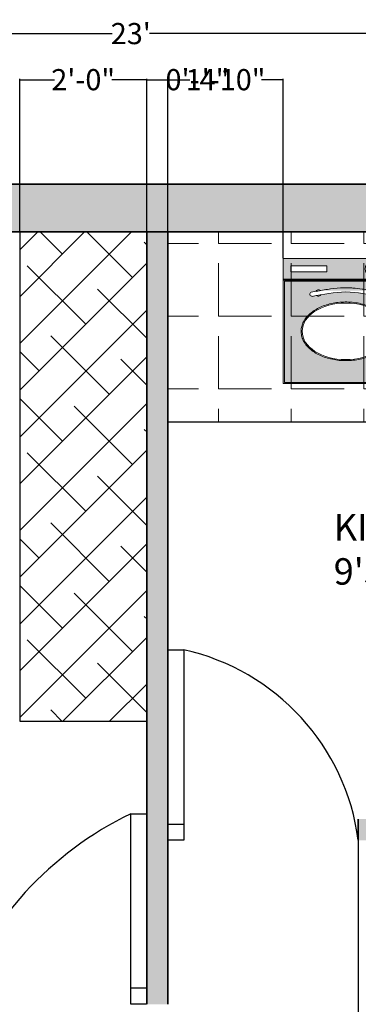
# Model space of a CAD drawing. Units: inches. Extents: x 490 to 851, y 299 to 716.
# Tile 3 of 3: x 664 to 728, y 530 to 716. Entities that reach past the tile are written whole.
import ezdxf

# ---------------------------------------------------------------- set-up
doc = ezdxf.new("R2010")
doc.units = ezdxf.units.IN
doc.header["$MEASUREMENT"] = 0
for name, color, linetype, lineweight in [('A-ANNO-DIMS', 2, 'Continuous', 18), ('A-AREA-IDEN', 7, 'Continuous', 25), ('A-DOOR', 3, 'Continuous', 25), ('A-EQPM', 8, 'Continuous', 18), ('A-EQPM-PATT', 9, 'Continuous', 13), ('A-FLOR-CASE', 40, 'Continuous', 25), ('A-FLOR-CASE-PATT', 9, 'Continuous', 13), ('A-WALL', 7, 'Continuous', 35), ('A-WALL-PATT', 1, 'Continuous', 13)]:
    doc.layers.add(name, color=color, linetype=linetype, lineweight=lineweight)
doc.styles.get("Standard").update_dxf_attribs({"font": 'arial.ttf'})
doc.dimstyles.get("Standard").update_dxf_attribs({"dimtxt": 4, "dimasz": 0.18, "dimexe": 0.18, "dimexo": 0.0625, "dimgap": 0.09, "dimtad": 0, "dimtih": 1, "dimtoh": 1, "dimdec": 0, "dimrnd": 6, "dimzin": 0, "dimdsep": 46, "dimlunit": 3, "dimtxsty": 'Standard', "dimcen": 0.09, "dimadec": 0, "dimazin": 0, "dimtfac": 1, "dimtdec": 0, "dimtofl": 0, "dimtmove": 0, "dimatfit": 3, "dimfxl": 1, "dimtolj": 1, "dimtzin": 0, "dimarcsym": 0})

# ---------------------------------------------------------------- blocks, each defined once
blk = doc.blocks.new('A$C7E884C79')
for p, q in [((-1.70119819813e-05, 1.5003966837e-05), (-1.70119419636e-05, 600.0000150039222)), ((-1.70119419636e-05, 600.0000150039222), (-1.70119819813e-05, 1.5003966837e-05)), ((-1.70119419636e-05, 600.0000150039222), (599.9999829879742, 600.0000150039077)), ((599.9999829879742, 600.0000150039077), (599.9999829880543, 1.5003966837e-05)), ((599.9999829880543, 1.5003966837e-05), (599.9999829879742, 600.0000150039077)), ((599.9999829879742, 600.0000150039077), (599.9999829879742, 450.0000150039659)), ((599.9999829879742, 600.0000150039077), (599.999982988058, 500.0000150039222)), ((599.999982988058, 500.0000150039222), (-1.70119383256e-05, 500.0000150039368)), ((599.999982988058, 495.0000150039441), (-1.70119019458e-05, 495.0000150039368)), ((599.999982988058, 500.0000150039222), (599.9999829880543, 1.5003966837e-05)), ((-1.70119819813e-05, 1.5003966837e-05), (599.9999829880543, 1.5003966837e-05))]:
    blk.add_line(p, q)
for points in [[(36.4219297853997, 564.739244228137), (208.9464086602384, 564.7392442281297), (208.9464086601583, 535.2607857798894), (36.4219297853997, 535.2607857798894)], [(4.999982988054398, 490.0000150040023), (594.999982988018, 490.0000150039513), (594.999982988018, 5.000015003966836), (4.999982987974362, 5.000015003930457)]]:
    blk.add_lwpolyline(points, close=True)
for centre, radius in [((419.341129777058, 550.0000150039514), 27.0465612830012), ((513.9038640534054, 550.0000150040095), 27.0465612830012), ((419.341129777058, 550.0000150039514), 17.0465612830012), ((513.9038640534054, 550.0000150040095), 17.0465612830012)]:
    blk.add_circle(centre, radius)
for centre, radius, start, end in [((137.2371143128039, 427.9571012842962), 9.99999999999936, 107.9829144627732, 276.9581094476087), ((168.4662399462322, 434.1738953022822), 14.99999999999999, 50.78880560725227, 150.3670062790382), ((168.4662399462322, 434.1738953022822), 14.99999999999999, 234.0164507050499, 327.1412143486447), ((431.5337276184946, 434.1738953023768), 14.99999999999999, 212.858785649389, 305.9835492949501), ((431.5337276184946, 434.1738953023768), 14.99999999999999, 29.63299372096182, 129.2111943927477), ((462.7628532516318, 427.957101284347), 9.99999999999936, 263.0418905523912, 72.01708553722673)]:
    blk.add_arc(centre, radius, start, end)
blk.add_ellipse((299.9999829880799, 250.0000150039296), major_axis=(-209.5453259160858, -5.8e-15), ratio=0.6483519184224599)
for points, knots in [([(134.1497789577479, 437.4685875095702), (144.6082166758169, 439.5062024863827), (155.1126203912208, 441.5529426086532), (185.9929094715517, 447.3437385568786), (206.494733029569, 450.9047119657725), (247.8674864836758, 456.3761860351832), (268.7408772092858, 458.286932131693), (293.5357101192494, 458.8504522635657), (297.2767330304487, 458.8901691064702), (304.7624299796444, 458.8727062536881), (308.4995762127364, 458.8160495901202), (319.6935092446511, 458.5127217792715), (327.132745431325, 458.1327232394569), (349.3790513168205, 456.541815341955), (364.1144689435605, 454.8805655177448), (399.790008761498, 449.8898845417889), (420.6328031065277, 446.1500348981672), (449.5099892856014, 440.6522069539087), (457.6940766911502, 439.0576405788188), (465.8501870183317, 437.4685875095119)], [0, 0, 0, 0, 31.63886493985545, 31.63886493985545, 92.6001428223882, 92.6001428223882, 153.561420704921, 153.561420704921, 164.3676472469802, 164.3676472469802, 175.1738737890395, 175.1738737890395, 196.786326873158, 196.786326873158, 240.011233041395, 240.011233041395, 302.0992006983722, 302.0992006983722, 326.7730650015291, 326.7730650015291, 326.7730650015291, 326.7730650015291]), ([(85.4546570720122, 250.000015003995), (85.45465707196854, 244.8170777658043), (85.88822561246344, 239.6342308201456), (88.02000493869853, 226.9220552357911), (90.21816192173355, 219.4365483580441), (96.38934370677816, 204.8396118246929), (100.3615888692657, 197.7281744404427), (109.949488846185, 184.0573372099134), (115.5648436689007, 177.4976038454224), (128.2787075515953, 165.0792487628459), (135.3771921305961, 159.2204529245464), (150.8720546014374, 148.3331296320939), (159.2684172301451, 143.3046103743872), (177.1485118738346, 134.1894280664528), (186.6321541176294, 130.1028504448732), (206.452394453896, 122.9637707452166), (216.7888352855625, 119.9113613978661), (238.0601333966843, 114.9105694415302), (248.9947899629697, 112.9622577759255), (271.1933164569673, 110.2148003270667), (282.4569621843111, 109.4156943254311), (305.0360465127196, 108.9852871540024), (316.3512522399324, 109.3539922337331), (338.7547296880475, 111.250649079022), (349.842772469201, 112.7785733309465), (371.5188673051307, 116.9582324470866), (382.1067079762179, 119.6099073260157), (402.521673323441, 125.9760737243086), (412.3486219806691, 129.6904786132982), (430.9992961862953, 138.0977836687561), (439.8229044345789, 142.7905902191232), (456.2471036538445, 153.0498538677457), (463.8476543751239, 158.616262825697), (477.6310685340795, 170.4997415048819), (483.8139313680366, 176.8169072710916), (494.5927765360757, 190.0604633081639), (499.1886010545786, 196.9871541335851), (506.6510537532812, 211.2839776396031), (509.5170666792983, 218.6543269104914), (513.4150547302415, 233.6388937332849), (514.4461961801352, 241.2525613148282), (514.6307693529524, 256.4928783461756), (513.7841458961847, 264.1183282945521), (510.2477897096396, 279.1482905806288), (507.5588601688614, 286.5521574531694), (500.4381704066108, 300.9341605102481), (496.0070741749878, 307.9124682590946), (485.5423204980033, 321.2743467604842), (479.5088542609591, 327.6582316730155), (466.0064121881987, 339.6881924907093), (458.5374402723464, 345.3343844510992), (442.356079099205, 355.7645443168249), (433.643722825036, 360.5484732858849), (415.1928234087136, 369.1474950443399), (405.4543904653837, 372.9624956318466), (385.1916535080673, 379.5371793190816), (374.6675208302404, 382.2967738713005), (353.0924824455687, 386.6971874674664), (342.0417855184496, 388.3379435140769), (319.6857084956864, 390.4625844960347), (308.380556257187, 390.9464386215868), (285.7940339416527, 390.7459687177425), (274.5128969021971, 390.0616475992965), (252.2522801997875, 387.5407311810659), (241.273026189534, 385.704172406523), (219.886530266871, 380.921302532438), (209.4794921704815, 377.9750595404139), (189.4937597145654, 371.0403800096638), (179.9152279588161, 367.0520348783057), (161.8232383307077, 358.1233102125143), (153.3098778178173, 353.1830191051149), (137.5613657555441, 342.4603322407738), (130.3262354594117, 336.6779568452357), (117.3219427482508, 324.3988645588861), (111.5527951950935, 317.9019950986867), (101.6427302403026, 304.3410831906103), (97.50207040229724, 297.2767107389691), (90.98281377420064, 282.7548846949166), (88.60495846102276, 275.2973569409469), (86.02335275324731, 261.8687924363285), (85.45465707200856, 255.934491795876), (85.4546570720122, 250.000015003995)], [0, 0, 0, 0, 0.1083005230516948, 0.1083005230516948, 0.2675342177864238, 0.2675342177864238, 0.4267679125211527, 0.4267679125211527, 0.5860016072558816, 0.5860016072558816, 0.7452353019906105, 0.7452353019906105, 0.9044689967253393, 0.9044689967253393, 1.063702691460068, 1.063702691460068, 1.222936386194797, 1.222936386194797, 1.382170080929526, 1.382170080929526, 1.541403775664254, 1.541403775664254, 1.700637470398983, 1.700637470398983, 1.859871165133712, 1.859871165133712, 2.019104859868441, 2.019104859868441, 2.17833855460317, 2.17833855460317, 2.337572249337898, 2.337572249337898, 2.496805944072627, 2.496805944072627, 2.656039638807356, 2.656039638807356, 2.815273333542085, 2.815273333542085, 2.974507028276814, 2.974507028276814, 3.133740723011543, 3.133740723011543, 3.292974417746271, 3.292974417746271, 3.452208112481, 3.452208112481, 3.611441807215729, 3.611441807215729, 3.770675501950458, 3.770675501950458, 3.929909196685187, 3.929909196685187, 4.089142891419916, 4.089142891419916, 4.248376586154645, 4.248376586154645, 4.407610280889374, 4.407610280889374, 4.566843975624102, 4.566843975624102, 4.726077670358831, 4.726077670358831, 4.88531136509356, 4.88531136509356, 5.044545059828289, 5.044545059828289, 5.203778754563018, 5.203778754563018, 5.363012449297746, 5.363012449297746, 5.522246144032475, 5.522246144032475, 5.681479838767204, 5.681479838767204, 5.840713533501933, 5.840713533501933, 5.999947228236662, 5.999947228236662, 6.15918092297139, 6.15918092297139, 6.283185307179586, 6.283185307179586, 6.283185307179586, 6.283185307179586])]:
    blk.add_open_spline(points, degree=3, knots=knots)
blk.add_open_spline([(137.9744605147498, 417.8376983042863), (191.9829680058602, 428.3601631990827), (299.999982988136, 449.4050929886863), (408.016997970407, 428.360163199051), (462.0255054615699, 417.837698304228)], degree=3)
blk = doc.blocks.new('*D102')
at = {"layer": 'A-ANNO-DIMS', "color": 0, "lineweight": -2, "transparency": 16777216}
for p, q in [((546.6878542437281, 685.0194991519433), (546.6878542437281, 713.5977998437985)), ((546.867854243728, 713.4177998437985), (681.1694777089394, 713.4177998437985)), ((822.507854243728, 713.4177998437985), (688.2062307785166, 713.4177998437985)), ((822.687854243728, 685.0194991519433), (822.687854243728, 713.5977998437985))]:
    blk.add_line(p, q, dxfattribs=at)
at = {"layer": 'A-ANNO-DIMS', "color": 0, "transparency": 16777216}
for points in [[(546.867854243728, 713.4477998437985), (546.867854243728, 713.3877998437985), (546.6878542437281, 713.4177998437985)], [(822.507854243728, 713.4477998437985), (822.507854243728, 713.3877998437985), (822.687854243728, 713.4177998437985)]]:
    blk.add_solid(points, dxfattribs=at)
at = {"layer": 'Defpoints', "color": 0, "transparency": 16777216}
for p in [(822.687854243728, 713.4177998437985), (546.6878542437281, 684.9569991519433), (822.687854243728, 684.9569991519433)]:
    blk.add_point(p, dxfattribs=at)
at = {"layer": 'A-ANNO-DIMS', "color": 0, "transparency": 16777216, "insert": (684.687854243728, 713.4177998437985), "char_height": 4, "attachment_point": 5}
blk.add_mtext("\\A1;23'", dxfattribs=at)
blk = doc.blocks.new('DOOR-LEAF-36IN')
blk.add_line((2.999854243728236, 2.99999915194337), (-0.0001457562717633, 2.99999915194337))
blk.add_lwpolyline([(-0.0001457562717633, -8.480566294e-07), (-0.0001457562717633, 35.99999915194337), (2.999854243728236, 35.99999915194337), (2.999854243728236, -8.480566294e-07)], close=True)
blk = doc.blocks.new('*D123')
at = {"layer": 'A-ANNO-DIMS', "color": 0, "lineweight": -2, "transparency": 16777216}
for p, q in [((663.687854, 676.019499), (663.687854, 704.886999)), ((663.8678539999999, 704.7069989999999), (670.247240084584, 704.7069989999999)), ((687.507854, 704.7069989999999), (681.1284679154161, 704.7069989999999)), ((687.6878539999999, 676.019499), (687.6878539999999, 704.886999))]:
    blk.add_line(p, q, dxfattribs=at)
at = {"layer": 'A-ANNO-DIMS', "color": 0, "transparency": 16777216}
for points in [[(663.8678539999999, 704.7369989999999), (663.8678539999999, 704.676999), (663.687854, 704.7069989999999)], [(687.507854, 704.7369989999999), (687.507854, 704.676999), (687.6878539999999, 704.7069989999999)]]:
    blk.add_solid(points, dxfattribs=at)
at = {"layer": 'Defpoints', "color": 0, "transparency": 16777216}
for p in [(687.6878539999999, 704.7069989999999), (663.687854, 675.956999), (687.6878539999999, 675.956999)]:
    blk.add_point(p, dxfattribs=at)
at = {"layer": 'A-ANNO-DIMS', "color": 0, "transparency": 16777216, "insert": (675.687854, 704.7069989999999), "char_height": 4, "attachment_point": 5}
blk.add_mtext('\\A1;2\'-0"', dxfattribs=at)
blk = doc.blocks.new('*D124')
at = {"layer": 'A-ANNO-DIMS', "color": 0, "lineweight": -2, "transparency": 16777216}
for p, q in [((687.6878539999999, 676.019499), (687.6878539999999, 704.886999)), ((687.867854, 704.7069989999999), (691.507854, 704.7069989999999)), ((691.6878539999999, 676.019499), (691.6878539999999, 704.886999)), ((691.6878539999999, 704.7069989999999), (691.867854, 704.7069989999999))]:
    blk.add_line(p, q, dxfattribs=at)
at = {"layer": 'A-ANNO-DIMS', "color": 0, "transparency": 16777216}
for points in [[(687.867854, 704.7369989999999), (687.867854, 704.676999), (687.6878539999999, 704.7069989999999)], [(691.507854, 704.7369989999999), (691.507854, 704.676999), (691.6878539999999, 704.7069989999999)]]:
    blk.add_solid(points, dxfattribs=at)
at = {"layer": 'Defpoints', "color": 0, "transparency": 16777216}
for p in [(691.6878539999999, 704.7069989999999), (687.6878539999999, 675.956999), (691.6878539999999, 675.956999)]:
    blk.add_point(p, dxfattribs=at)
at = {"layer": 'A-ANNO-DIMS', "color": 0, "transparency": 16777216, "insert": (697.2743615034105, 704.7069989999999), "char_height": 4, "attachment_point": 5}
blk.add_mtext('\\A1;0\'-4"', dxfattribs=at)
blk = doc.blocks.new('*D141')
at = {"layer": 'A-ANNO-DIMS', "color": 0, "lineweight": -2, "transparency": 16777216}
for p, q in [((691.6878539999999, 676.019499), (691.6878539999999, 704.886999)), ((691.867854, 704.7069989999999), (695.8265687598908, 704.7069989999999)), ((713.32954, 704.7069989999999), (709.3708252401092, 704.7069989999999)), ((713.5095399999999, 670.98891), (713.5095399999999, 704.886999))]:
    blk.add_line(p, q, dxfattribs=at)
at = {"layer": 'A-ANNO-DIMS', "color": 0, "transparency": 16777216}
for points in [[(691.867854, 704.7369989999999), (691.867854, 704.676999), (691.6878539999999, 704.7069989999999)], [(713.32954, 704.7369989999999), (713.32954, 704.676999), (713.5095399999999, 704.7069989999999)]]:
    blk.add_solid(points, dxfattribs=at)
at = {"layer": 'Defpoints', "color": 0, "transparency": 16777216}
for p in [(713.5095399999999, 704.7069989999999), (691.6878539999999, 675.956999), (713.5095399999999, 670.92641)]:
    blk.add_point(p, dxfattribs=at)
at = {"layer": 'A-ANNO-DIMS', "color": 0, "transparency": 16777216, "insert": (702.5986969999999, 704.7069989999999), "char_height": 4, "attachment_point": 5}
blk.add_mtext('\\A1;1\'-10"', dxfattribs=at)
blk = doc.blocks.new('*D143')
at = {"layer": 'A-ANNO-DIMS', "color": 0, "lineweight": -2, "transparency": 16777216}
for p, q in [((727.687854, 560.894499), (727.687854, 304.927739)), ((777.687854, 560.894499), (777.687854, 304.927739)), ((727.8678539999999, 305.107739), (747.2008553642565, 305.107739)), ((777.507854, 305.107739), (758.1748526357435, 305.107739))]:
    blk.add_line(p, q, dxfattribs=at)
at = {"layer": 'A-ANNO-DIMS', "color": 0, "transparency": 16777216}
for points in [[(727.8678539999999, 305.1377389999999), (727.8678539999999, 305.077739), (727.687854, 305.107739)], [(777.507854, 305.1377389999999), (777.507854, 305.077739), (777.687854, 305.107739)]]:
    blk.add_solid(points, dxfattribs=at)
at = {"layer": 'Defpoints', "color": 0, "transparency": 16777216}
for p in [(727.687854, 560.9569989999999), (777.687854, 560.9569989999999), (777.687854, 305.107739)]:
    blk.add_point(p, dxfattribs=at)
at = {"layer": 'A-ANNO-DIMS', "color": 0, "transparency": 16777216, "insert": (752.687854, 305.107739), "char_height": 4, "attachment_point": 5}
blk.add_mtext('\\A1;4\'-2"', dxfattribs=at)

msp = doc.modelspace()

# ---------------------------------------------------------------- hatches: boundary and pattern name
at = {"layer": 'A-EQPM-PATT'}
h = msp.add_hatch(color=256, dxfattribs=at)
h.dxf.hatch_style = 1
edge = h.paths.add_edge_path(flags=0)
edge.add_ellipse((725.3205634423474, 657.1468827041818), major_axis=(8.249815980948258, 3.137e-13), ratio=0.648351918422466, start_angle=0, end_angle=360)
edge = h.paths.add_edge_path(flags=0)
edge.add_ellipse((748.9426106864386, 657.1468827041818), major_axis=(8.249815980948258, 3.137e-13), ratio=0.648351918422466, start_angle=0, end_angle=360)
h.paths.add_polyline_path([(760.5567839147827, 666.5957016018205), (737.3284374580912, 666.5957016018225), (737.328437458088, 647.5012134128433), (760.5567839147827, 647.5012134128445)])
edge = h.paths.add_edge_path(flags=16)
edge.add_spline(control_points=[(740.4959443117903, 657.1468827041843), (740.4959443117887, 656.9428300570115), (740.513013939367, 656.7387809646627), (740.5969422592976, 656.238301610948), (740.683483872803, 655.943596615761), (740.9264437855999, 655.368914075078), (741.0828313904223, 655.0889362253043), (741.4603077674664, 654.5507142870945), (741.6813847289907, 654.2924570680201), (742.181930551144, 653.8035454505958), (742.461398447955, 653.5728841971194), (743.0714324035, 653.1442494218261), (743.4019978613231, 652.9462762227037), (744.1059385953266, 652.5874107775095), (744.4793103372083, 652.4265218947702), (745.259634759896, 652.1454557648624), (745.6665812493317, 652.0252821685099), (746.5040339308719, 651.8284005954259), (746.934532220883, 651.7516954117406), (747.8084899568673, 651.6435277956438), (748.251940576054, 651.6120669294378), (749.1408809039442, 651.5951217652083), (749.5863614443855, 651.6096377132291), (750.4683881155711, 651.6843092425713), (750.9049252329394, 651.7444637406785), (751.758314793409, 651.9090172491879), (752.1751589143181, 652.0134138979646), (752.9788977075159, 652.2640503703385), (753.3657854499264, 652.4102867832906), (754.1000639619589, 652.7412830453165), (754.4474501134661, 652.926039208717), (755.0940721299727, 653.3299472263792), (755.393306410338, 653.5490971853537), (755.9359605110842, 654.0169506766601), (756.1793803076966, 654.2656579902905), (756.6037442906904, 654.7870578342696), (756.7846822638598, 655.0597621974754), (757.0784796142024, 655.6226292646414), (757.1913147687701, 655.9128004957787), (757.344778865264, 656.5027440714792), (757.3853749853384, 656.802494763666), (757.3926416456854, 657.4025072452151), (757.3593100135294, 657.7027218101118), (757.2200833920119, 658.2944526087763), (757.1142200242647, 658.5859434305298), (756.8338779076405, 659.152164023328), (756.6594253000964, 659.4269005488733), (756.2474271238373, 659.9529587575895), (756.0098890830087, 660.204292809264), (755.4782968754197, 660.6779133138975), (755.1842428629845, 660.9002043359601), (754.5471813994751, 661.310840551146), (754.2041752469486, 661.4991842113454), (753.4777618841014, 661.8377283750641), (753.0943590123167, 661.987925248588), (752.2966134628161, 662.246771063046), (751.8822775306182, 662.3554165178577), (751.0328665705918, 662.5286611476281), (750.5977997624374, 662.5932578423766), (749.7176392497302, 662.6769051251308), (749.2725545159311, 662.6959545001525), (748.3833213539021, 662.6880619842531), (747.9391821003803, 662.6611202079364), (747.0627798680019, 662.5618715300532), (746.63052577311, 662.4895660664885), (745.7885377446587, 662.3012641029419), (745.378811835352, 662.1852702843584), (744.591971974883, 661.912251405195), (744.214864425444, 661.7552299433305), (743.5025813692192, 661.403705350189), (743.1674096954835, 661.2092057002914), (742.5473895355515, 660.7870526741362), (742.2625418860974, 660.5594000995088), (741.750561858099, 660.0759712693376), (741.5234300646675, 659.820189007125), (741.1332700270774, 659.2862948375157), (740.9702519232188, 659.0081699378447), (740.7135882764434, 658.4364445030395), (740.6199719255308, 658.1428410481587), (740.5183339055397, 657.6141574062448), (740.4959443117901, 657.3805235227624), (740.4959443117903, 657.1468827041843)], knot_values=[0, 0, 0, 0, 0.1083005230516948, 0.1083005230516948, 0.2675342177864238, 0.2675342177864238, 0.4267679125211527, 0.4267679125211527, 0.5860016072558816, 0.5860016072558816, 0.7452353019906105, 0.7452353019906105, 0.9044689967253393, 0.9044689967253393, 1.063702691460068, 1.063702691460068, 1.222936386194797, 1.222936386194797, 1.382170080929526, 1.382170080929526, 1.541403775664254, 1.541403775664254, 1.700637470398983, 1.700637470398983, 1.859871165133712, 1.859871165133712, 2.019104859868441, 2.019104859868441, 2.17833855460317, 2.17833855460317, 2.337572249337898, 2.337572249337898, 2.496805944072627, 2.496805944072627, 2.656039638807356, 2.656039638807356, 2.815273333542085, 2.815273333542085, 2.974507028276814, 2.974507028276814, 3.133740723011543, 3.133740723011543, 3.292974417746271, 3.292974417746271, 3.452208112481, 3.452208112481, 3.611441807215729, 3.611441807215729, 3.770675501950458, 3.770675501950458, 3.929909196685187, 3.929909196685187, 4.089142891419916, 4.089142891419916, 4.248376586154645, 4.248376586154645, 4.407610280889374, 4.407610280889374, 4.566843975624102, 4.566843975624102, 4.726077670358831, 4.726077670358831, 4.88531136509356, 4.88531136509356, 5.044545059828289, 5.044545059828289, 5.203778754563018, 5.203778754563018, 5.363012449297746, 5.363012449297746, 5.522246144032475, 5.522246144032475, 5.681479838767204, 5.681479838767204, 5.840713533501933, 5.840713533501933, 5.999947228236662, 5.999947228236662, 6.15918092297139, 6.15918092297139, 6.283185307179586, 6.283185307179586, 6.283185307179586, 6.283185307179586], degree=3, periodic=0)
edge = h.paths.add_edge_path(flags=0)
edge.add_ellipse((748.9426106864386, 657.1468827041818), major_axis=(8.249815980948258, 3.137e-13), ratio=0.648351918422466, start_angle=0, end_angle=360)
edge = h.paths.add_edge_path(flags=16)
edge.add_spline(control_points=[(742.4130750946933, 664.5275351650338), (742.6914882918603, 664.5817783431816), (742.9707288907302, 664.6361857766777), (743.2508036674241, 664.6898164654069)], knot_values=[0, 0, 0, 0, 21.39329177210675, 21.39329177210675, 21.39329177210675, 21.39329177210675], degree=3, periodic=0)
edge.add_arc((743.7641168658934, 664.3978228734082), 0.5905511811023694, 50.78880560234279, 150.3670062825767, ccw=False)
edge.add_spline(control_points=[(744.1374519240431, 664.8553943233596), (744.779067646516, 664.97139206178), (745.4250780596886, 665.0781755879807), (746.8901501941393, 665.2719288077744), (747.7119372305805, 665.3471550320465), (748.688111754595, 665.36934086401), (748.8353961211775, 665.3709045192425), (749.1301085994924, 665.3702170053534), (749.2772403409527, 665.3679864280476), (749.7179463658312, 665.3560443882504), (750.0108296802672, 665.3410838158167), (750.8866684946568, 665.2784496466238), (751.4668030468905, 665.2130461102375), (752.8713518586205, 665.0165626072471), (753.6919343131492, 664.8693244323014), (754.8288314068135, 664.6528745132362), (755.1510395723863, 664.5900963094923), (755.4721462781808, 664.5275351650314)], knot_values=[43.89785635095746, 43.89785635095746, 43.89785635095746, 43.89785635095746, 92.6001428223882, 92.6001428223882, 153.561420704921, 153.561420704921, 164.3676472469802, 164.3676472469802, 175.1738737890395, 175.1738737890395, 196.786326873158, 196.786326873158, 240.011233041395, 240.011233041395, 302.0992006983722, 302.0992006983722, 326.7730650015291, 326.7730650015291, 326.7730650015291, 326.7730650015291], degree=3, periodic=0)
edge.add_arc((754.1211045695258, 664.397822873412), 0.5905511811023695, 29.64555569566221, 129.3131094229314, ccw=False)
edge.add_spline(control_points=[(744.1374519240431, 664.8553943233596), (744.779067646516, 664.97139206178), (745.4250780596886, 665.0781755879807), (746.8901501941393, 665.2719288077744), (747.7119372305805, 665.3471550320465), (748.688111754595, 665.36934086401), (748.8353961211775, 665.3709045192425), (749.1301085994924, 665.3702170053534), (749.2772403409527, 665.3679864280476), (749.7179463658312, 665.3560443882504), (750.0108296802672, 665.3410838158167), (750.8866684946568, 665.2784496466238), (751.4668030468905, 665.2130461102375), (752.8713518586205, 665.0165626072471), (753.6919343131492, 664.8693244323014), (754.8288314068135, 664.6528745132362), (755.1510395723863, 664.5900963094923), (755.4721462781808, 664.5275351650314)], knot_values=[43.89785635095746, 43.89785635095746, 43.89785635095746, 43.89785635095746, 92.6001428223882, 92.6001428223882, 153.561420704921, 153.561420704921, 164.3676472469802, 164.3676472469802, 175.1738737890395, 175.1738737890395, 196.786326873158, 196.786326873158, 240.011233041395, 240.011233041395, 302.0992006983722, 302.0992006983722, 326.7730650015291, 326.7730650015291, 326.7730650015291, 326.7730650015291], degree=3, periodic=0)
edge.add_arc((755.3505977046888, 664.1530672034108), 0.3937007874015679, -101.0087676412142, 72.01708553236932, ccw=False)
edge.add_spline(control_points=[(755.3215682641351, 663.7546655112802), (755.037073723253, 663.810093516205), (754.7525791823709, 663.8655215211298), (754.4680846414888, 663.9199572781217)], knot_values=[304.9124823041715, 304.9124823041715, 304.9124823041715, 304.9124823041715, 326.7730650015789, 326.7730650015789, 326.7730650015789, 326.7730650015789], degree=3, periodic=0)
edge.add_arc((754.1211045695258, 664.397822873412), 0.5905511811023683, 212.8587871331284, 305.9835477310444, ccw=False)
edge.add_spline(control_points=[(753.6250354635439, 664.0774073001456), (752.0642272045088, 664.3599897262603), (748.9426107100477, 664.8064223787223), (745.8209942155868, 664.3599897330135), (744.2601859801605, 664.0774073129695)], knot_values=[43.45390602737222, 43.45390602737222, 43.45390602737222, 43.45390602737222, 163.3865343148396, 283.3191607881738, 283.3191607881738, 283.3191607881738, 283.3191607881738], degree=3, periodic=0)
edge.add_arc((743.7641168658934, 664.3978228734082), 0.5905511811023553, 234.01645070441748, 327.1412143484826, ccw=False)
edge.add_spline(control_points=[(743.417136780882, 663.9199572875928), (743.1326422235041, 663.8655215275596), (742.8481476661264, 663.8100935194209), (742.5636531087486, 663.7546655112824)], knot_values=[0, 0, 0, 0, 21.86058396493695, 21.86058396493695, 21.86058396493695, 21.86058396493695], degree=3, periodic=0)
edge.add_arc((742.5346237307191, 664.1530672034088), 0.393700787401568, 107.9829001472302, 281.00876763934195, ccw=False)
h.paths.add_polyline_path([(736.9347366706914, 666.5957016018205), (713.706390214, 666.5957016018225), (713.7063902139969, 647.5012134128433), (736.9347366706914, 647.5012134128445)])
edge = h.paths.add_edge_path(flags=16)
edge.add_spline(control_points=[(716.8738970676992, 657.1468827041843), (716.8738970676975, 656.9428300570115), (716.8909666952759, 656.7387809646627), (716.9748950152064, 656.238301610948), (717.0614366287118, 655.943596615761), (717.3043965415088, 655.368914075078), (717.4607841463312, 655.0889362253043), (717.8382605233752, 654.5507142870945), (718.0593374848995, 654.2924570680201), (718.5598833070528, 653.8035454505958), (718.8393512038638, 653.5728841971194), (719.4493851594088, 653.1442494218261), (719.7799506172319, 652.9462762227037), (720.4838913512355, 652.5874107775095), (720.8572630931171, 652.4265218947702), (721.6375875158049, 652.1454557648624), (722.0445340052405, 652.0252821685099), (722.8819866867807, 651.8284005954259), (723.312484976792, 651.7516954117406), (724.1864427127762, 651.6435277956438), (724.6298933319629, 651.6120669294378), (725.518833659853, 651.5951217652083), (725.9643142002944, 651.6096377132291), (726.84634087148, 651.6843092425713), (727.2828779888483, 651.7444637406785), (728.136267549318, 651.9090172491879), (728.5531116702269, 652.0134138979646), (729.3568504634247, 652.2640503703385), (729.7437382058351, 652.4102867832906), (730.4780167178678, 652.7412830453165), (730.825402869375, 652.926039208717), (731.4720248858815, 653.3299472263792), (731.7712591662468, 653.5490971853537), (732.3139132669932, 654.0169506766601), (732.5573330636055, 654.2656579902905), (732.9816970465993, 654.7870578342696), (733.1626350197686, 655.0597621974754), (733.4564323701113, 655.6226292646414), (733.5692675246789, 655.9128004957787), (733.7227316211728, 656.5027440714792), (733.7633277412472, 656.802494763666), (733.7705944015944, 657.4025072452151), (733.7372627694382, 657.7027218101118), (733.5980361479207, 658.2944526087763), (733.4921727801734, 658.5859434305298), (733.2118306635494, 659.152164023328), (733.0373780560052, 659.4269005488733), (732.6253798797461, 659.9529587575895), (732.3878418389176, 660.204292809264), (731.8562496313285, 660.6779133138975), (731.5621956188934, 660.9002043359601), (730.925134155384, 661.310840551146), (730.5821280028575, 661.4991842113454), (729.8557146400102, 661.8377283750641), (729.4723117682256, 661.987925248588), (728.6745662187249, 662.246771063046), (728.2602302865271, 662.3554165178577), (727.4108193265005, 662.5286611476281), (726.9757525183463, 662.5932578423766), (726.0955920056391, 662.6769051251308), (725.65050727184, 662.6959545001525), (724.761274109811, 662.6880619842531), (724.317134856289, 662.6611202079364), (723.4407326239107, 662.5618715300532), (723.0084785290189, 662.4895660664885), (722.1664905005676, 662.3012641029419), (721.7567645912609, 662.1852702843584), (720.9699247307918, 661.912251405195), (720.5928171813528, 661.7552299433305), (719.880534125128, 661.403705350189), (719.5453624513922, 661.2092057002914), (718.9253422914603, 660.7870526741362), (718.6404946420062, 660.5594000995088), (718.1285146140078, 660.0759712693376), (717.9013828205763, 659.820189007125), (717.5112227829862, 659.2862948375157), (717.3482046791275, 659.0081699378447), (717.0915410323522, 658.4364445030395), (716.9979246814397, 658.1428410481587), (716.8962866614485, 657.6141574062448), (716.8738970676989, 657.3805235227624), (716.8738970676992, 657.1468827041843)], knot_values=[0, 0, 0, 0, 0.1083005230516948, 0.1083005230516948, 0.2675342177864238, 0.2675342177864238, 0.4267679125211527, 0.4267679125211527, 0.5860016072558816, 0.5860016072558816, 0.7452353019906105, 0.7452353019906105, 0.9044689967253393, 0.9044689967253393, 1.063702691460068, 1.063702691460068, 1.222936386194797, 1.222936386194797, 1.382170080929526, 1.382170080929526, 1.541403775664254, 1.541403775664254, 1.700637470398983, 1.700637470398983, 1.859871165133712, 1.859871165133712, 2.019104859868441, 2.019104859868441, 2.17833855460317, 2.17833855460317, 2.337572249337898, 2.337572249337898, 2.496805944072627, 2.496805944072627, 2.656039638807356, 2.656039638807356, 2.815273333542085, 2.815273333542085, 2.974507028276814, 2.974507028276814, 3.133740723011543, 3.133740723011543, 3.292974417746271, 3.292974417746271, 3.452208112481, 3.452208112481, 3.611441807215729, 3.611441807215729, 3.770675501950458, 3.770675501950458, 3.929909196685187, 3.929909196685187, 4.089142891419916, 4.089142891419916, 4.248376586154645, 4.248376586154645, 4.407610280889374, 4.407610280889374, 4.566843975624102, 4.566843975624102, 4.726077670358831, 4.726077670358831, 4.88531136509356, 4.88531136509356, 5.044545059828289, 5.044545059828289, 5.203778754563018, 5.203778754563018, 5.363012449297746, 5.363012449297746, 5.522246144032475, 5.522246144032475, 5.681479838767204, 5.681479838767204, 5.840713533501933, 5.840713533501933, 5.999947228236662, 5.999947228236662, 6.15918092297139, 6.15918092297139, 6.283185307179586, 6.283185307179586, 6.283185307179586, 6.283185307179586], degree=3, periodic=0)
edge = h.paths.add_edge_path(flags=0)
edge.add_ellipse((725.3205634423474, 657.1468827041818), major_axis=(8.249815980948258, 3.137e-13), ratio=0.648351918422466, start_angle=0, end_angle=360)
edge = h.paths.add_edge_path(flags=16)
edge.add_spline(control_points=[(731.6995210200438, 663.7546655112802), (731.4150264791617, 663.810093516205), (731.1305319382795, 663.8655215211298), (730.8460373973976, 663.9199572781217)], knot_values=[304.9124823041715, 304.9124823041715, 304.9124823041715, 304.9124823041715, 326.7730650015789, 326.7730650015789, 326.7730650015789, 326.7730650015789], degree=3, periodic=0)
edge.add_arc((730.4990573254347, 664.397822873412), 0.5905511811023683, 212.8587871331377, 305.9835477310444, ccw=False)
edge.add_spline(control_points=[(730.0029882194526, 664.0774073001456), (728.4421799604175, 664.3599897262603), (725.3205634659566, 664.8064223787223), (722.1989469714956, 664.3599897330135), (720.6381387360695, 664.0774073129695)], knot_values=[43.45390602737222, 43.45390602737222, 43.45390602737222, 43.45390602737222, 163.3865343148396, 283.3191607881738, 283.3191607881738, 283.3191607881738, 283.3191607881738], degree=3, periodic=0)
edge.add_arc((720.1420696218023, 664.3978228734082), 0.5905511811023554, 234.01645070441748, 327.14121434847334, ccw=False)
edge.add_spline(control_points=[(719.7950895367909, 663.9199572875928), (719.5105949794131, 663.8655215275596), (719.2261004220353, 663.8100935194209), (718.9416058646574, 663.7546655112824)], knot_values=[0, 0, 0, 0, 21.86058396493695, 21.86058396493695, 21.86058396493695, 21.86058396493695], degree=3, periodic=0)
edge.add_arc((718.9125764866279, 664.1530672034088), 0.393700787401568, 107.9829001472302, 281.00876763934195, ccw=False)
edge.add_spline(control_points=[(718.7910278506022, 664.5275351650338), (719.0694410477691, 664.5817783431816), (719.3486816466392, 664.6361857766777), (719.628756423333, 664.6898164654069)], knot_values=[0, 0, 0, 0, 21.39329177210675, 21.39329177210675, 21.39329177210675, 21.39329177210675], degree=3, periodic=0)
edge.add_arc((720.1420696218023, 664.3978228734082), 0.5905511811023695, 50.78880560234978, 150.3670062825767, ccw=False)
edge.add_spline(control_points=[(720.5154046799519, 664.8553943233596), (721.1570204024248, 664.97139206178), (721.8030308155975, 665.0781755879807), (723.268102950048, 665.2719288077744), (724.0898899864894, 665.3471550320465), (725.0660645105037, 665.36934086401), (725.2133488770864, 665.3709045192425), (725.5080613554012, 665.3702170053534), (725.6551930968615, 665.3679864280476), (726.0958991217401, 665.3560443882504), (726.388782436176, 665.3410838158167), (727.2646212505655, 665.2784496466238), (727.8447558027995, 665.2130461102375), (729.2493046145294, 665.0165626072471), (730.069887069058, 664.8693244323014), (731.2067841627223, 664.6528745132362), (731.5289923282951, 664.5900963094923), (731.8500990340896, 664.5275351650314)], knot_values=[43.89785635095746, 43.89785635095746, 43.89785635095746, 43.89785635095746, 92.6001428223882, 92.6001428223882, 153.561420704921, 153.561420704921, 164.3676472469802, 164.3676472469802, 175.1738737890395, 175.1738737890395, 196.786326873158, 196.786326873158, 240.011233041395, 240.011233041395, 302.0992006983722, 302.0992006983722, 326.7730650015291, 326.7730650015291, 326.7730650015291, 326.7730650015291], degree=3, periodic=0)
edge.add_arc((730.4990573254347, 664.397822873412), 0.5905511811023695, 29.64555569566221, 129.3131094229314, ccw=False)
edge.add_spline(control_points=[(720.5154046799519, 664.8553943233596), (721.1570204024248, 664.97139206178), (721.8030308155975, 665.0781755879807), (723.268102950048, 665.2719288077744), (724.0898899864894, 665.3471550320465), (725.0660645105037, 665.36934086401), (725.2133488770864, 665.3709045192425), (725.5080613554012, 665.3702170053534), (725.6551930968615, 665.3679864280476), (726.0958991217401, 665.3560443882504), (726.388782436176, 665.3410838158167), (727.2646212505655, 665.2784496466238), (727.8447558027995, 665.2130461102375), (729.2493046145294, 665.0165626072471), (730.069887069058, 664.8693244323014), (731.2067841627223, 664.6528745132362), (731.5289923282951, 664.5900963094923), (731.8500990340896, 664.5275351650314)], knot_values=[43.89785635095746, 43.89785635095746, 43.89785635095746, 43.89785635095746, 92.6001428223882, 92.6001428223882, 153.561420704921, 153.561420704921, 164.3676472469802, 164.3676472469802, 175.1738737890395, 175.1738737890395, 196.786326873158, 196.786326873158, 240.011233041395, 240.011233041395, 302.0992006983722, 302.0992006983722, 326.7730650015291, 326.7730650015291, 326.7730650015291, 326.7730650015291], degree=3, periodic=0)
edge.add_arc((731.7285504605976, 664.1530672034108), 0.393700787401568, -101.0087676412142, 72.01708553236932, ccw=False)
h.paths.add_polyline_path([(737.1315870643906, 670.9264102632361), (713.5095398202994, 670.9264102632366), (713.5095398202992, 666.9894023892214), (737.131587064391, 666.9894023892209)])
h.paths.add_polyline_path([(728.954208541008, 668.9579063262299, -1), (731.0838590357325, 668.9579063262299, -1)], flags=16)
h.paths.add_polyline_path([(729.3479093284096, 668.9579063262299, -1), (730.6901582483309, 668.9579063262299, -1)], flags=0)
h.paths.add_polyline_path([(721.7357770514844, 668.3776217111093), (714.9434747335805, 668.3776217111093), (714.9434747335805, 669.5381909413553), (721.7357770514876, 669.538190941355)], flags=16)
h.paths.add_polyline_path([(732.6771508353524, 668.9579063262321, -1), (734.806801330077, 668.9579063262321, -1)], flags=16)
h.paths.add_polyline_path([(733.070851622754, 668.9579063262321, -1), (734.4131005426754, 668.9579063262321, -1)], flags=0)
h.paths.add_polyline_path([(760.7536343084817, 670.9264102632361), (737.1315870643906, 670.9264102632366), (737.131587064391, 666.9894023892214), (760.7536343084823, 666.9894023892209)])
h.paths.add_polyline_path([(752.5762557850992, 668.9579063262299, -1), (754.7059062798236, 668.9579063262299, -1)], flags=16)
h.paths.add_polyline_path([(745.3578242955756, 668.3776217111093), (738.5655219776717, 668.3776217111093), (738.5655219776717, 669.5381909413553), (745.3578242955788, 669.538190941355)], flags=16)
h.paths.add_polyline_path([(754.3122054924221, 668.9579063262299, -1), (752.9699565725008, 668.9579063262299, -1)], flags=0)
h.paths.add_polyline_path([(758.4288485741681, 668.9579063262321, -1), (756.2991980794436, 668.9579063262321, -1)], flags=16)
h.paths.add_polyline_path([(758.0351477867665, 668.9579063262321, -1), (756.6928988668451, 668.9579063262321, -1)], flags=0)
at = {"layer": 'A-FLOR-CASE-PATT'}
h = msp.add_hatch(dxfattribs=at)
h.set_pattern_fill('ANSI38', color=256, scale=50)
h.set_pattern_definition([(45, (0, 0), (-4.419417382415922, 4.419417382415922), []), (135, (0, 0), (-13.25825214724776, 4.419417382415923), [15.625, -9.375])])
h.paths.add_polyline_path([(687.6878542437281, 675.9569991519433), (663.6878542437281, 675.9569991519433), (663.6878542437281, 583.4645873544328), (687.6878542437282, 583.4645873544328)])
h.paths.add_polyline_path([(813.687854243728, 461.9569991519433), (747.0641290993162, 461.9569991519433), (747.0641290993162, 437.9569991519433), (813.687854243728, 437.9569991519433)])
h = msp.add_hatch(dxfattribs=at)
h.set_pattern_fill('ANGLE', color=256, scale=50)
h.set_pattern_definition([(0, (0, 0), (0, 13.75), [10, -3.75]), (90, (0, 0), (-13.75, 8e-16), [10, -3.75])])
h.paths.add_polyline_path([(813.687854243728, 675.9569991519433), (691.6878542437281, 675.9569991519433), (691.6878542437281, 639.9569991519435), (777.6878542437281, 639.9569991519434), (777.6878542437279, 600.9569991519433), (813.6878542437278, 600.9569991519433)])
at = {"layer": 'A-WALL-PATT'}
h = msp.add_hatch(color=256, dxfattribs=at)
h.dxf.hatch_style = 1
h.paths.add_polyline_path([(555.6878542437281, 497.9569991519433), (611.6878542437282, 497.9569991519434), (611.6878542437281, 493.9569991519433), (615.6878542437281, 493.9569991519433), (615.6878542437281, 501.9569991519433), (555.6878542437281, 501.9569991519433), (555.6878542437281, 529.9569991519433), (651.6878542437281, 529.9569991519433), (651.6878542437281, 533.9569991519433), (555.6878542437281, 533.9569991519433), (555.6878542437281, 675.9569991519433), (813.687854243728, 675.9569991519433), (813.6878542437278, 564.9569991519431), (813.6878542437278, 560.9569991519431), (813.6878542437278, 533.9569991519433), (802.5034207310172, 533.9569991519433), (802.5034207310172, 529.9569991519433), (813.687854243728, 529.9569991519433), (813.687854243728, 465.9569991519433), (727.6878542437282, 465.9569991519433), (727.6878542437282, 461.9569991519433), (813.687854243728, 461.9569991519433), (813.687854243728, 333.9569991519434), (786.3863959033706, 333.9569991519434), (786.3863959033706, 324.9569991519434), (822.687854243728, 324.9569991519434), (822.687854243728, 684.9569991519433), (546.6878542437281, 684.9569991519433), (546.6878542437281, 324.9569991519434), (555.7079255371355, 324.9569991519434), (555.7079255371355, 333.9569991519433), (555.6878542437281, 333.9569991519433), (555.6878542437281, 461.9569991519433), (651.6878542437282, 461.9569991519433), (651.6878542437282, 465.9569991519433), (555.6878542437281, 465.9569991519433)])
h.paths.add_polyline_path([(714.3863959033706, 333.9569991519433), (691.6878542437281, 333.9569991519433), (691.6878542437282, 429.9205150877742), (691.6792956389427, 429.9205150877742), (691.6792956389427, 465.9569991519433), (687.6878542437282, 465.9569991519433), (687.6878542437282, 429.9569991519434), (687.6878542437281, 361.0075905803756), (687.6936932778153, 361.0075905803756), (687.6936932778153, 324.9569991519434), (714.3863959033706, 324.9569991519434)], flags=17)
h.paths.add_polyline_path([(691.6878542437281, 675.9569991519433), (687.6878542437281, 675.9569991519433), (687.6878542437282, 529.9569991519433), (691.6878542437282, 529.9569991519433)], flags=17)
h.paths.add_polyline_path([(777.7575047331366, 533.9569991519433), (761.6878542437282, 533.9569991519433), (761.6878542437282, 497.9569991519433, -0.0312398925164955), (765.6878542437281, 498.2098446269331), (765.6878542437281, 529.9569991519433), (777.7575047331366, 529.9569991519433)], flags=17)
h.paths.add_polyline_path([(777.6878542437279, 564.9569991519434), (727.687854243728, 564.9569991519433), (727.687854243728, 560.9569991519434), (777.6878542437279, 560.9569991519434)], flags=17)

# ---------------------------------------------------------------- linework, layer by layer
at = {"layer": 'A-DOOR'}
for centre, radius, start, end in [((685.4872415957941, 555.3981042246706), 42.56516205388415, 7.504108928705974, 77.51678522729537), ((713.5941603641406, 506.3948125261148), 66.23871508464357, 115.8958901853617, 159.1626525884847)]:
    msp.add_arc(centre, radius, start, end, dxfattribs=at)
at = {"layer": 'A-FLOR-CASE'}
for p, q in [((663.6878542437281, 675.9569991519433), (663.6878542437281, 583.4645873544328)), ((777.6878542437282, 639.9569991519434), (691.6878542437281, 639.9569991519435)), ((663.6878542437282, 583.4645873544328), (687.6878542437282, 583.4645873544328))]:
    msp.add_line(p, q, dxfattribs=at)
at = {"layer": 'A-WALL'}
for p, q in [((822.687854243728, 684.9569991519433), (546.6878542437281, 684.9569991519433)), ((813.687854243728, 675.9569991519433), (555.6878542437281, 675.9569991519433)), ((687.6878542437281, 675.9569991519433), (687.6878542437282, 529.9569991519434)), ((691.6878542437281, 675.9569991519433), (691.6878542437282, 529.9569991519433)), ((727.687854243728, 564.9569991519431), (727.687854243728, 560.9569991519434))]:
    msp.add_line(p, q, dxfattribs=at)

# ---------------------------------------------------------------- block references
at = {"layer": 'A-DOOR'}
for p in [(691.6879999999999, 560.9569999999999), (684.6653910462034, 529.982440015059)]:
    msp.add_blockref('DOOR-LEAF-36IN', p, dxfattribs=at)
at = {"layer": 'A-EQPM', "xscale": 0.0393700787401575, "yscale": 0.0393700787401575, "zscale": 0.0393700787401575}
msp.add_blockref('A$C7E884C79', (713.5095404900608, 647.3043624284365), dxfattribs=at)

# ---------------------------------------------------------------- texts
at = {"layer": 'A-AREA-IDEN', "insert": (723.0449506801868, 622.59746330636), "char_height": 5, "attachment_point": 1}
msp.add_mtext_dynamic_manual_height_columns('KITCHEN\\P9\'3" x 7\'', width=54.99209744262703, gutter_width=1, heights=[0], dxfattribs=at)

# ---------------------------------------------------------------- dimensions: what is measured, and where the dimension line sits
at = {"layer": 'A-ANNO-DIMS'}
for base, p1, p2, override, picture, middle in [((822.687854243728, 713.4177998437985), (546.6878542437281, 684.9569991519433), (822.687854243728, 684.9569991519433), {"dimclrd": 0, "dimclre": 0, "dimclrt": 0}, '*D102', (684.687854243728, 713.4177998437985)), ((687.6878539999999, 704.7069989999999), (663.687854, 675.956999), (687.6878539999999, 675.956999), {"dimdec": 1, "dimlfac": 1, "dimrnd": 0, "dimzin": 1, "dimdsep": 46, "dimlunit": 4, "dimfrac": 2}, '*D123', (675.687854, 704.7069989999999)), ((691.6878539999999, 704.7069989999999), (687.6878539999999, 675.956999), (691.6878539999999, 675.956999), {"dimdec": 1, "dimlfac": 1, "dimrnd": 0, "dimzin": 1, "dimdsep": 46, "dimlunit": 4, "dimfrac": 2}, '*D124', (697.2743615034105, 704.7069989999999)), ((713.5095399999999, 704.7069989999999), (691.6878539999999, 675.956999), (713.5095399999999, 670.92641), {"dimdec": 1, "dimlfac": 1, "dimrnd": 0, "dimzin": 1, "dimdsep": 46, "dimlunit": 4, "dimfrac": 2}, '*D141', (702.5986969999999, 704.7069989999999)), ((777.687854, 305.107739), (727.687854, 560.9569989999999), (777.687854, 560.9569989999999), {"dimdec": 1, "dimlfac": 1, "dimrnd": 0, "dimzin": 1, "dimdsep": 46, "dimlunit": 4, "dimfrac": 2}, '*D143', (752.687854, 305.107739))]:
    dim = msp.add_linear_dim(base=base, p1=p1, p2=p2, dimstyle='Standard', override=override, dxfattribs=at)
    dim.commit()
    dim.dimension.update_dxf_attribs({"geometry": picture, "text_midpoint": middle})

doc.saveas('drawing.dxf')
